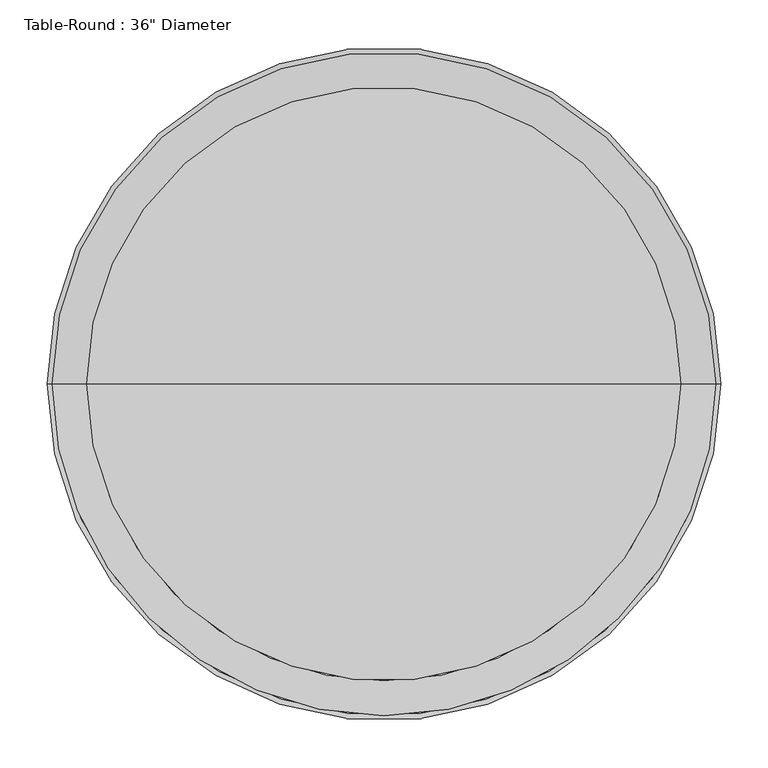
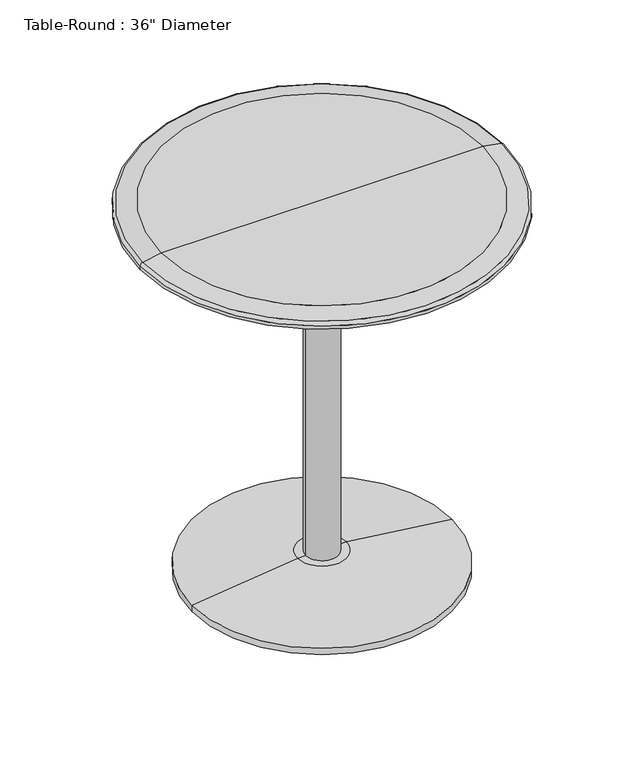
"""IFC4 building model written with IfcOpenShell, lengths in millimetres: furniture geometry."""

from ifc_helpers import new_model, si_unit, point, frame, origin, origin_2d, place, context, project, spatial, polyline, circle_curve, ellipse_curve, trimmed, segment, composite_curve, outline, extrude, source, transform, mapped, element, save
from ifc_brep_helpers import plane_surface, cylinder_surface, revolved_surface, advanced_brep


def furniture_a7e4c93f(model_context):
    return source(origin(), model_context, "Body", "SolidModel", [
        extrude(outline(composite_curve([segment(trimmed(circle_curve(origin_2d(), 31.75), [point((-31.75, 0.0))], [point((31.75, 0.0))], False, "CARTESIAN"), True, "CONTINUOUS"), segment(trimmed(circle_curve(origin_2d(), 31.75), [point((31.75, 0.0))], [point((-31.75, 0.0))], False, "CARTESIAN"), True, "CONTINUOUS")], self_intersect=False)), frame((0.0, 0.0, 38.1), z_axis=(0.0, 0.0, 1.0), x_axis=(1.0, 0.0, 0.0)), (0.0, 0.0, 1.0), 704.85),
        advanced_brep(
        [(0.0, 0.0, 742.95), (-355.6, 0.0, 742.95), (355.6, 0.0, 742.95), (313.7011364, 0.0, 762.0), (-313.7011364, 0.0, 762.0), (0.0, 0.0, 762.0), (350.3526659, 0.0, 755.5373465), (-350.3526659, 0.0, 755.5373465), (355.6, 0.0, 749.2838172), (-355.6, 0.0, 749.2838172)],
        [
            (0, 1),
            (1, 2, circle_curve(frame((0.0, 0.0, 742.95), z_axis=(0.0, 0.0, -1.0), x_axis=(-1.0, 0.0, 0.0)), 355.6)),
            (2, 0),
            (2, 1, circle_curve(frame((0.0, 0.0, 742.95), z_axis=(0.0, 0.0, -1.0), x_axis=(-1.0, 0.0, 0.0)), 355.6)),
            (3, 4, circle_curve(frame((0.0, 0.0, 762.0), z_axis=(0.0, 0.0, 1.0), x_axis=(-1.0, 0.0, 0.0)), 313.7011364)),
            (4, 5),
            (5, 3),
            (4, 3, circle_curve(frame((0.0, 0.0, 762.0), z_axis=(0.0, 0.0, 1.0), x_axis=(-1.0, 0.0, 0.0)), 313.7011364)),
            (6, 7, circle_curve(frame((0.0, 0.0, 755.5373465), z_axis=(0.0, 0.0, 1.0), x_axis=(-1.0, 0.0, 0.0)), 350.3526659)),
            (7, 4),
            (3, 6),
            (7, 6, circle_curve(frame((0.0, 0.0, 755.5373465), z_axis=(0.0, 0.0, 1.0), x_axis=(-1.0, 0.0, 0.0)), 350.3526659)),
            (8, 9, circle_curve(frame((0.0, 0.0, 749.2838172), z_axis=(0.0, 0.0, 1.0), x_axis=(-1.0, 0.0, 0.0)), 355.6)),
            (9, 7, circle_curve(frame((-349.25, 0.0, 749.2838172), z_axis=(0.0, 1.0, 0.0), x_axis=(1.0, 0.0, 0.0)), 6.35)),
            (6, 8, circle_curve(frame((349.25, 0.0, 749.2838172), z_axis=(0.0, 1.0, 0.0), x_axis=(-1.0, 0.0, 0.0)), 6.35)),
            (9, 8, circle_curve(frame((0.0, 0.0, 749.2838172), z_axis=(0.0, 0.0, 1.0), x_axis=(-1.0, 0.0, 0.0)), 355.6)),
            (1, 9),
            (8, 2),
        ],
        [
            plane_surface(frame((0.0, 0.0, 742.95), z_axis=(0.0, 0.0, -1.0), x_axis=(-1.0, 0.0, 0.0))),
            plane_surface(frame((0.0, 0.0, 762.0), z_axis=(0.0, 0.0, 1.0), x_axis=(-1.0, 0.0, 0.0))),
            revolved_surface(polyline([(-313.7011364, 0.0, 762.0), (-350.3526659, 0.0, 755.5373465)]), (0.0, 0.0, 838.2), (0.0, 0.0, -1.0)),
            revolved_surface(trimmed(ellipse_curve(frame((-349.25, 0.0, 749.2838172), z_axis=(0.0, -1.0, 0.0), x_axis=(1.0, 0.0, 0.0)), 6.35, 6.35), [point((-350.3526659, 0.0, 755.5373465))], [point((-355.6, 0.0, 749.2838172))], True, "CARTESIAN"), (0.0, 0.0, 838.2), (0.0, 0.0, -1.0)),
            cylinder_surface(frame((0.0, 0.0, 838.2), z_axis=(0.0, 0.0, -1.0), x_axis=(-1.0, 0.0, 0.0)), 355.6),
        ],
        [
            (0, [[1, 2, 3]]),
            (0, [[-3, 4, -1]]),
            (1, [[5, 6, 7]]),
            (1, [[8, -7, -6]]),
            (2, [[9, 10, -5, 11]]),
            (2, [[12, -11, -8, -10]]),
            (3, [[13, 14, -9, 15]]),
            (3, [[16, -15, -12, -14]]),
            (4, [[-2, 17, -13, 18]]),
            (4, [[-4, -18, -16, -17]]),
        ],
    ),
        advanced_brep(
        [(0.0, 0.0, 0.0), (-254.0, 0.0, 0.0), (254.0, 0.0, 0.0), (47.625, 0.0, 38.1), (-47.625, 0.0, 38.1), (0.0, 0.0, 38.1), (254.0, 0.0, 12.7), (-254.0, 0.0, 12.7)],
        [
            (0, 1),
            (1, 2, circle_curve(frame((0.0, 0.0, 0.0), z_axis=(0.0, 0.0, -1.0), x_axis=(-1.0, 0.0, 0.0)), 254.0)),
            (2, 0),
            (2, 1, circle_curve(frame((0.0, 0.0, 0.0), z_axis=(0.0, 0.0, -1.0), x_axis=(-1.0, 0.0, 0.0)), 254.0)),
            (3, 4, circle_curve(frame((0.0, 0.0, 38.1), z_axis=(0.0, 0.0, 1.0), x_axis=(-1.0, 0.0, 0.0)), 47.625)),
            (4, 5),
            (5, 3),
            (4, 3, circle_curve(frame((0.0, 0.0, 38.1), z_axis=(0.0, 0.0, 1.0), x_axis=(-1.0, 0.0, 0.0)), 47.625)),
            (6, 7, circle_curve(frame((0.0, 0.0, 12.7), z_axis=(0.0, 0.0, 1.0), x_axis=(-1.0, 0.0, 0.0)), 254.0)),
            (7, 4),
            (3, 6),
            (7, 6, circle_curve(frame((0.0, 0.0, 12.7), z_axis=(0.0, 0.0, 1.0), x_axis=(-1.0, 0.0, 0.0)), 254.0)),
            (1, 7),
            (6, 2),
        ],
        [
            plane_surface(frame((0.0, 0.0, 0.0), z_axis=(0.0, 0.0, -1.0), x_axis=(-1.0, 0.0, 0.0))),
            plane_surface(frame((0.0, 0.0, 38.1), z_axis=(0.0, 0.0, 1.0), x_axis=(-1.0, 0.0, 0.0))),
            revolved_surface(polyline([(-47.625, 0.0, 38.1), (-254.0, 0.0, 12.7)]), (0.0, 0.0, 215.9), (0.0, 0.0, -1.0)),
            cylinder_surface(frame((0.0, 0.0, 215.9), z_axis=(0.0, 0.0, -1.0), x_axis=(-1.0, 0.0, 0.0)), 254.0),
        ],
        [
            (0, [[1, 2, 3]]),
            (0, [[-3, 4, -1]]),
            (1, [[5, 6, 7]]),
            (1, [[8, -7, -6]]),
            (2, [[9, 10, -5, 11]]),
            (2, [[12, -11, -8, -10]]),
            (3, [[-2, 13, -9, 14]]),
            (3, [[-4, -14, -12, -13]]),
        ],
    ),
    ])


if __name__ == "__main__":
    model = new_model("IFC4")
    model_context = context("Model", 3, world=origin())
    ifc_project = project(units=[si_unit("LENGTHUNIT", "METRE", prefix="MILLI")], contexts=[model_context])
    site = spatial("IfcSite", under=ifc_project)
    building = spatial("IfcBuilding", under=site)
    placement = place(None, origin())
    furniture_shape = furniture_a7e4c93f(model_context)
    element("IfcFurniture", 1, ObjectType="Table-Round : 36\" Diameter", at=placement, inside=building, context=model_context, shape_type="MappedRepresentation", body=[
        mapped(furniture_shape, transform((0.0, 0.0, 0.0), x_axis=(1.0, 0.0, 0.0), y_axis=(0.0, 1.0, 0.0), z_axis=(0.0, 0.0, 1.0))),
    ])
    save(model, "model.ifc")

# Revit data of these elements
# Type "Table-Round : 36\" Diameter"
#   Assembly Code = "E2020200"
#   Base Radius = 0' - 10"
#   Height = 2' - 6"
#   Radius = 1' - 2"
#   Base Material = Steel, Chrome Plated
#   Top Material = Birch
#   Default Elevation = 0
# Element 1 (IfcFurniture, "Table-Round : 36\" Diameter")
#   Materials on its faces: "Steel, Chrome Plated", "Birch"
# Materials
#   "Steel, Chrome Plated": class "Metal", colour RGB 17 17 17, transparency 0, Description = "Chromiuim plated steel", Cost = 0
#   "Birch": class "Wood", colour RGB 224 178 126, transparency 0, Description = "Betula Alleghaniensis", Cost = 0
